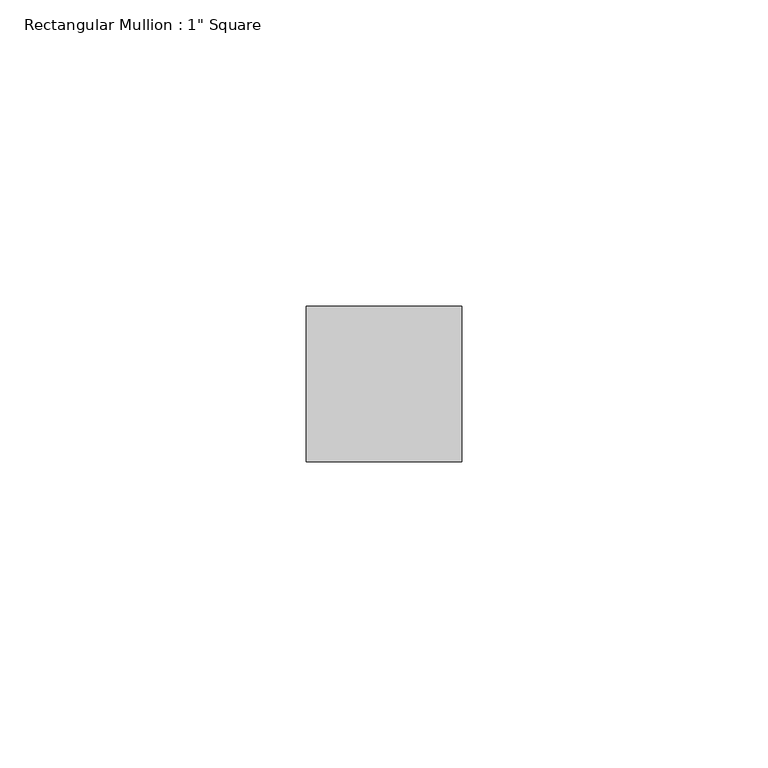
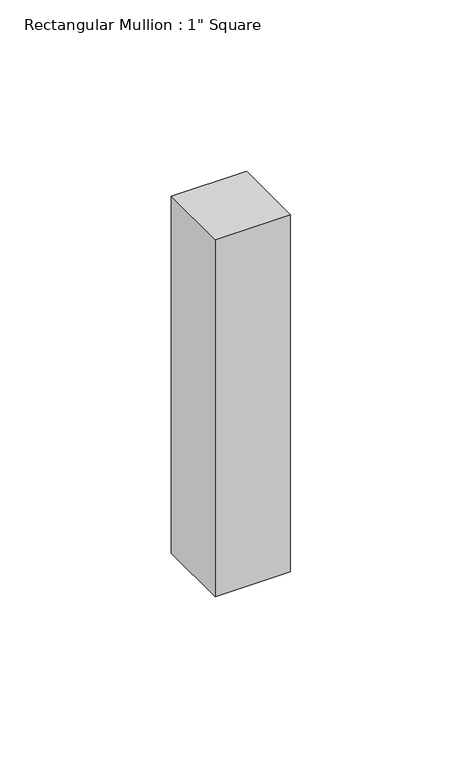
"""IFC4 building model written with IfcOpenShell, lengths in millimetres: member geometry."""

from ifc_helpers import new_model, si_unit, frame, origin, place, context, project, spatial, polyline, outline, extrude, source, transform, mapped, element, save


def member_4ec4fa50(model_context):
    return source(origin(), model_context, "Body", "SweptSolid", [
        extrude(outline(polyline([(0.0, 12.7), (0.0, -12.7), (-25.4, -12.7), (-25.4, 12.7), (0.0, 12.7)])), frame((0.0, 0.0, -127.0), z_axis=(0.0, 0.0, 1.0), x_axis=(1.0, 0.0, 0.0)), (0.0, 0.0, 1.0), 127.0),
    ])


if __name__ == "__main__":
    model = new_model("IFC4")
    model_context = context("Model", 3, world=origin())
    ifc_project = project(units=[si_unit("LENGTHUNIT", "METRE", prefix="MILLI")], contexts=[model_context])
    site = spatial("IfcSite", under=ifc_project)
    building = spatial("IfcBuilding", under=site)
    placement = place(None, origin())
    member_shape = member_4ec4fa50(model_context)
    element("IfcMember", 1, ObjectType="Rectangular Mullion : 1\" Square", at=placement, inside=building, context=model_context, shape_type="MappedRepresentation", body=[
        mapped(member_shape, transform((0.0, 0.0, 0.0), x_axis=(1.0, 0.0, 0.0), y_axis=(0.0, 1.0, 0.0), z_axis=(0.0, 0.0, 1.0))),
    ])
    save(model, "model.ifc")

# Revit data of these elements
# Type "Rectangular Mullion : 1\" Square"
#   built-in parameter 1007304 = 0.0833333 (stored number, unit not read)
#   built-in parameter 1007301 = 0.0416667 (stored number, unit not read)
#   built-in parameter 1007300 = 0.0416667 (stored number, unit not read)
